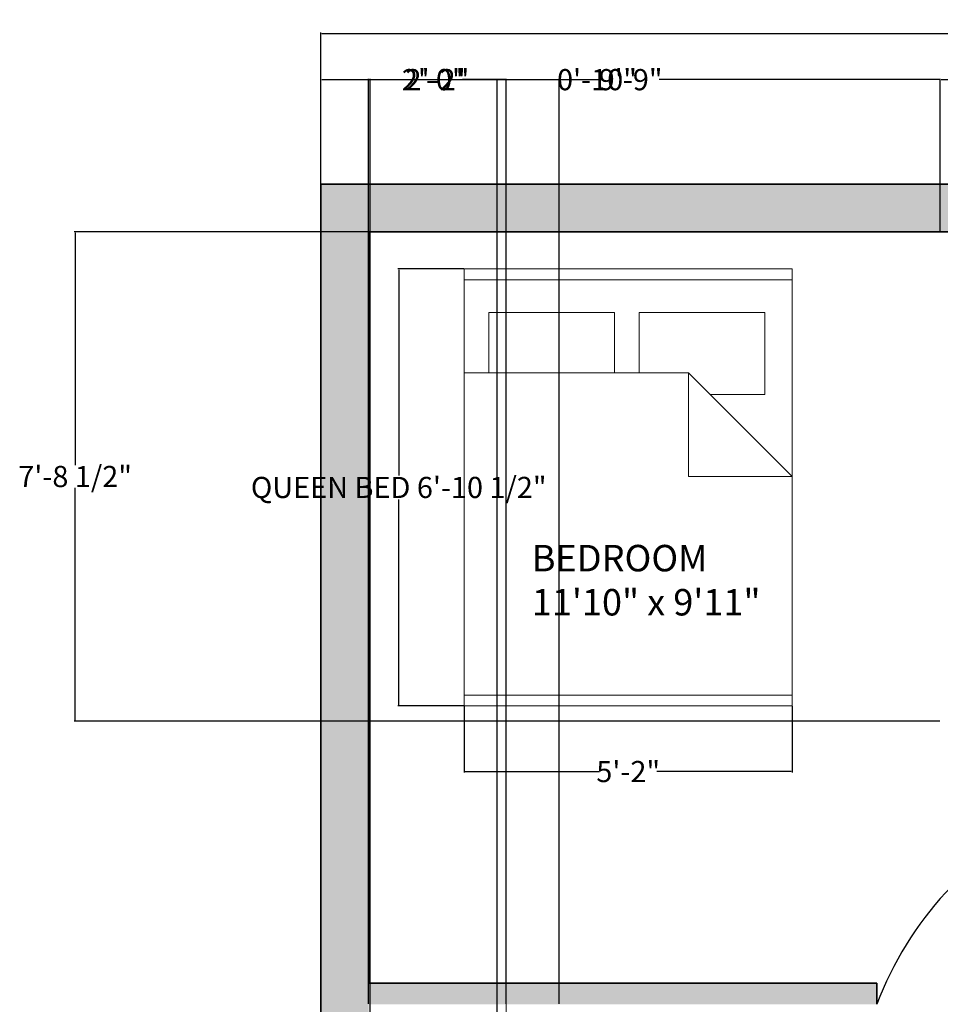
# Model space of a CAD drawing. Units: inches. Extents: x 490 to 851, y 299 to 716.
# Tile 2 of 3: x 490 to 664, y 530 to 716. Entities that reach past the tile are written whole.
import ezdxf

# ---------------------------------------------------------------- set-up
doc = ezdxf.new("R2010")
doc.units = ezdxf.units.IN
doc.header["$MEASUREMENT"] = 0
for name, color, linetype, lineweight in [('A-ANNO-DIMS', 2, 'Continuous', 18), ('A-AREA-IDEN', 7, 'Continuous', 25), ('A-DOOR', 3, 'Continuous', 25), ('A-WALL', 7, 'Continuous', 35), ('A-WALL-PATT', 1, 'Continuous', 13), ('beds', 40, 'Continuous', 18), ('stairs', 82, 'Continuous', 18)]:
    doc.layers.add(name, color=color, linetype=linetype, lineweight=lineweight)
doc.styles.get("Standard").update_dxf_attribs({"font": 'arial.ttf'})
doc.dimstyles.get("Standard").update_dxf_attribs({"dimtxt": 4, "dimasz": 0.18, "dimexe": 0.18, "dimexo": 0.0625, "dimgap": 0.09, "dimtad": 0, "dimtih": 1, "dimtoh": 1, "dimdec": 0, "dimrnd": 6, "dimzin": 0, "dimdsep": 46, "dimlunit": 3, "dimtxsty": 'Standard', "dimcen": 0.09, "dimadec": 0, "dimazin": 0, "dimtfac": 1, "dimtdec": 0, "dimtofl": 0, "dimtmove": 0, "dimatfit": 3, "dimfxl": 1, "dimtolj": 1, "dimtzin": 0, "dimarcsym": 0})

# ---------------------------------------------------------------- blocks, each defined once
blk = doc.blocks.new('QUEEN-00')
for p, q in [((-0.8475, -0.7751), (-0.8475, 0.7489)), ((0.6511, 0.7489), (0.6511, -0.2925)), ((1.0829, 0.7489), (1.0829, -0.7751)), ((0.9305, 0.6346), (0.6511, 0.6346)), ((0.9305, 0.0504), (0.9305, 0.6346)), ((0.6511, 0.0504), (0.9305, 0.0504)), ((0.9305, -0.0639), (0.6511, -0.0639)), ((0.9305, -0.6481), (0.9305, -0.0639)), ((0.1685, -0.7751), (0.6511, -0.2925)), ((0.1685, -0.2925), (0.1685, -0.7751)), ((0.6511, -0.2925), (0.1685, -0.2925)), ((0.5495, -0.3941), (0.5495, -0.6481)), ((0.5495, -0.6481), (0.9305, -0.6481))]:
    blk.add_line(p, q)
blk.add_lwpolyline([(-0.8983, -0.7751), (-0.8983, 0.7489), (1.1337, 0.7489), (1.1337, -0.7751)], close=True)
blk = doc.blocks.new('*D102')
at = {"layer": 'A-ANNO-DIMS', "color": 0, "lineweight": -2, "transparency": 16777216}
for p, q in [((546.69, 685.02), (546.69, 713.6)), ((546.87, 713.42), (681.17, 713.42)), ((822.51, 713.42), (688.21, 713.42)), ((822.69, 685.02), (822.69, 713.6))]:
    blk.add_line(p, q, dxfattribs=at)
at = {"layer": 'A-ANNO-DIMS', "color": 0, "transparency": 16777216}
for points in [[(546.87, 713.45), (546.87, 713.39), (546.69, 713.42)], [(822.51, 713.45), (822.51, 713.39), (822.69, 713.42)]]:
    blk.add_solid(points, dxfattribs=at)
at = {"layer": 'Defpoints', "color": 0, "transparency": 16777216}
for p in [(822.69, 713.42), (546.69, 684.96), (822.69, 684.96)]:
    blk.add_point(p, dxfattribs=at)
at = {"layer": 'A-ANNO-DIMS', "color": 0, "transparency": 16777216, "insert": (684.69, 713.42), "char_height": 4, "attachment_point": 5}
blk.add_mtext("\\A1;23'", dxfattribs=at)
blk = doc.blocks.new('*D112')
at = {"layer": 'A-ANNO-DIMS', "color": 0, "lineweight": -2, "transparency": 16777216}
for p, q in [((573.7, 668.93), (561.2, 668.93)), ((561.38, 668.75), (561.38, 629.92)), ((561.38, 586.52), (561.38, 625.36)), ((573.7, 586.34), (561.2, 586.34))]:
    blk.add_line(p, q, dxfattribs=at)
at = {"layer": 'A-ANNO-DIMS', "color": 0, "transparency": 16777216}
for points in [[(561.35, 668.75), (561.41, 668.75), (561.38, 668.93)], [(561.35, 586.52), (561.41, 586.52), (561.38, 586.34)]]:
    blk.add_solid(points, dxfattribs=at)
at = {"layer": 'Defpoints', "color": 0, "transparency": 16777216}
for p in [(561.38, 668.93), (573.77, 668.93), (573.77, 586.34)]:
    blk.add_point(p, dxfattribs=at)
at = {"layer": 'A-ANNO-DIMS', "color": 0, "transparency": 16777216, "insert": (561.38, 627.64), "char_height": 4, "attachment_point": 5}
blk.add_mtext('\\A1;QUEEN BED 6\'-10 1/2"', dxfattribs=at)
blk = doc.blocks.new('*D113')
at = {"layer": 'A-ANNO-DIMS', "color": 0, "lineweight": -2, "transparency": 16777216}
for p, q in [((573.77, 586.28), (573.77, 573.77)), ((635.71, 586.28), (635.71, 573.77)), ((573.95, 573.95), (599.33, 573.95)), ((635.53, 573.95), (610.15, 573.95))]:
    blk.add_line(p, q, dxfattribs=at)
at = {"layer": 'A-ANNO-DIMS', "color": 0, "transparency": 16777216}
for points in [[(573.95, 573.98), (573.95, 573.92), (573.77, 573.95)], [(635.53, 573.98), (635.53, 573.92), (635.71, 573.95)]]:
    blk.add_solid(points, dxfattribs=at)
at = {"layer": 'Defpoints', "color": 0, "transparency": 16777216}
for p in [(573.77, 586.34), (635.71, 586.34), (573.77, 573.95)]:
    blk.add_point(p, dxfattribs=at)
at = {"layer": 'A-ANNO-DIMS', "color": 0, "transparency": 16777216, "insert": (604.74, 573.95), "char_height": 4, "attachment_point": 5}
blk.add_mtext('\\A1;5\'-2"', dxfattribs=at)
blk = doc.blocks.new('*D122')
at = {"layer": 'A-ANNO-DIMS', "color": 0, "lineweight": -2, "transparency": 16777216}
for p, q in [((546.69, 685.02), (546.69, 704.89)), ((546.87, 704.71), (599.78, 704.71)), ((663.51, 704.71), (610.59, 704.71)), ((663.69, 676.02), (663.69, 704.89))]:
    blk.add_line(p, q, dxfattribs=at)
at = {"layer": 'A-ANNO-DIMS', "color": 0, "transparency": 16777216}
for points in [[(546.87, 704.74), (546.87, 704.68), (546.69, 704.71)], [(663.51, 704.74), (663.51, 704.68), (663.69, 704.71)]]:
    blk.add_solid(points, dxfattribs=at)
at = {"layer": 'Defpoints', "color": 0, "transparency": 16777216}
for p in [(663.69, 704.71), (546.69, 684.96), (663.69, 675.96)]:
    blk.add_point(p, dxfattribs=at)
at = {"layer": 'A-ANNO-DIMS', "color": 0, "transparency": 16777216, "insert": (605.19, 704.71), "char_height": 4, "attachment_point": 5}
blk.add_mtext('\\A1;9\'-9"', dxfattribs=at)
blk = doc.blocks.new('*D123')
at = {"layer": 'A-ANNO-DIMS', "color": 0, "lineweight": -2, "transparency": 16777216}
for p, q in [((663.69, 676.02), (663.69, 704.89)), ((663.87, 704.71), (670.25, 704.71)), ((687.51, 704.71), (681.13, 704.71)), ((687.69, 676.02), (687.69, 704.89))]:
    blk.add_line(p, q, dxfattribs=at)
at = {"layer": 'A-ANNO-DIMS', "color": 0, "transparency": 16777216}
for points in [[(663.87, 704.74), (663.87, 704.68), (663.69, 704.71)], [(687.51, 704.74), (687.51, 704.68), (687.69, 704.71)]]:
    blk.add_solid(points, dxfattribs=at)
at = {"layer": 'Defpoints', "color": 0, "transparency": 16777216}
for p in [(687.69, 704.71), (663.69, 675.96), (687.69, 675.96)]:
    blk.add_point(p, dxfattribs=at)
at = {"layer": 'A-ANNO-DIMS', "color": 0, "transparency": 16777216, "insert": (675.69, 704.71), "char_height": 4, "attachment_point": 5}
blk.add_mtext('\\A1;2\'-0"', dxfattribs=at)
blk = doc.blocks.new('*D125')
at = {"layer": 'A-ANNO-DIMS', "color": 0, "lineweight": -2, "transparency": 16777216}
for p, q in [((663.63, 675.96), (500.07, 675.96)), ((500.25, 675.78), (500.25, 631.87)), ((500.25, 583.64), (500.25, 627.55)), ((663.63, 583.46), (500.07, 583.46))]:
    blk.add_line(p, q, dxfattribs=at)
at = {"layer": 'A-ANNO-DIMS', "color": 0, "transparency": 16777216}
for points in [[(500.22, 675.78), (500.28, 675.78), (500.25, 675.96)], [(500.22, 583.64), (500.28, 583.64), (500.25, 583.46)]]:
    blk.add_solid(points, dxfattribs=at)
at = {"layer": 'Defpoints', "color": 0, "transparency": 16777216}
for p in [(500.25, 675.96), (663.69, 675.96), (663.69, 583.46)]:
    blk.add_point(p, dxfattribs=at)
at = {"layer": 'A-ANNO-DIMS', "color": 0, "transparency": 16777216, "insert": (500.25, 629.71), "char_height": 4, "attachment_point": 5}
blk.add_mtext('\\A1;7\'-8 1/2"', dxfattribs=at)
blk = doc.blocks.new('*D131')
at = {"layer": 'A-ANNO-DIMS', "color": 0, "lineweight": -2, "transparency": 16777216}
for p, q in [((555.69, 530.02), (555.69, 704.89)), ((555.87, 704.71), (563.25, 704.71)), ((581.51, 704.71), (574.13, 704.71)), ((581.69, 530.02), (581.69, 704.89))]:
    blk.add_line(p, q, dxfattribs=at)
at = {"layer": 'A-ANNO-DIMS', "color": 0, "transparency": 16777216}
for points in [[(555.87, 704.74), (555.87, 704.68), (555.69, 704.71)], [(581.51, 704.74), (581.51, 704.68), (581.69, 704.71)]]:
    blk.add_solid(points, dxfattribs=at)
at = {"layer": 'Defpoints', "color": 0, "transparency": 16777216}
for p in [(581.69, 704.71), (555.69, 529.96), (581.69, 529.96)]:
    blk.add_point(p, dxfattribs=at)
at = {"layer": 'A-ANNO-DIMS', "color": 0, "transparency": 16777216, "insert": (568.69, 704.71), "char_height": 4, "attachment_point": 5}
blk.add_mtext('\\A1;2\'-2"', dxfattribs=at)
blk = doc.blocks.new('*D132')
at = {"layer": 'A-ANNO-DIMS', "color": 0, "lineweight": -2, "transparency": 16777216}
for p, q in [((581.69, 530.02), (581.69, 704.89)), ((581.87, 704.71), (591.51, 704.71)), ((591.69, 530.02), (591.69, 704.89)), ((591.69, 704.71), (591.87, 704.71))]:
    blk.add_line(p, q, dxfattribs=at)
at = {"layer": 'A-ANNO-DIMS', "color": 0, "transparency": 16777216}
for points in [[(581.87, 704.74), (581.87, 704.68), (581.69, 704.71)], [(591.51, 704.74), (591.51, 704.68), (591.69, 704.71)]]:
    blk.add_solid(points, dxfattribs=at)
at = {"layer": 'Defpoints', "color": 0, "transparency": 16777216}
for p in [(591.69, 704.71), (581.69, 529.96), (591.69, 529.96)]:
    blk.add_point(p, dxfattribs=at)
at = {"layer": 'A-ANNO-DIMS', "color": 0, "transparency": 16777216, "insert": (598.83, 704.71), "char_height": 4, "attachment_point": 5}
blk.add_mtext('\\A1;0\'-10"', dxfattribs=at)
blk = doc.blocks.new('*D136')
at = {"layer": 'A-ANNO-DIMS', "color": 0, "lineweight": -2, "transparency": 16777216}
for p, q in [((556, 494.66), (556, 704.89)), ((556.18, 704.71), (562.56, 704.71)), ((579.82, 704.71), (573.44, 704.71)), ((580, 490.16), (580, 704.89))]:
    blk.add_line(p, q, dxfattribs=at)
at = {"layer": 'A-ANNO-DIMS', "color": 0, "transparency": 16777216}
for points in [[(556.18, 704.74), (556.18, 704.68), (556, 704.71)], [(579.82, 704.74), (579.82, 704.68), (580, 704.71)]]:
    blk.add_solid(points, dxfattribs=at)
at = {"layer": 'Defpoints', "color": 0, "transparency": 16777216}
for p in [(580, 704.71), (556, 494.6), (580, 490.1)]:
    blk.add_point(p, dxfattribs=at)
at = {"layer": 'A-ANNO-DIMS', "color": 0, "transparency": 16777216, "insert": (568, 704.71), "char_height": 4, "attachment_point": 5}
blk.add_mtext('\\A1;2\'-0"', dxfattribs=at)

msp = doc.modelspace()

# ---------------------------------------------------------------- hatches: boundary and pattern name
at = {"layer": 'A-WALL-PATT'}
h = msp.add_hatch(color=256, dxfattribs=at)
h.dxf.hatch_style = 1
h.paths.add_polyline_path([(555.69, 497.96), (611.69, 497.96), (611.69, 493.96), (615.69, 493.96), (615.69, 501.96), (555.69, 501.96), (555.69, 529.96), (651.69, 529.96), (651.69, 533.96), (555.69, 533.96), (555.69, 675.96), (813.69, 675.96), (813.69, 564.96), (813.69, 560.96), (813.69, 533.96), (802.5, 533.96), (802.5, 529.96), (813.69, 529.96), (813.69, 465.96), (727.69, 465.96), (727.69, 461.96), (813.69, 461.96), (813.69, 333.96), (786.39, 333.96), (786.39, 324.96), (822.69, 324.96), (822.69, 684.96), (546.69, 684.96), (546.69, 324.96), (555.71, 324.96), (555.71, 333.96), (555.69, 333.96), (555.69, 461.96), (651.69, 461.96), (651.69, 465.96), (555.69, 465.96)])
h.paths.add_polyline_path([(714.39, 333.96), (691.69, 333.96), (691.69, 429.92), (691.68, 429.92), (691.68, 465.96), (687.69, 465.96), (687.69, 429.96), (687.69, 361.01), (687.69, 361.01), (687.69, 324.96), (714.39, 324.96)], flags=17)
h.paths.add_polyline_path([(691.69, 675.96), (687.69, 675.96), (687.69, 529.96), (691.69, 529.96)], flags=17)
h.paths.add_polyline_path([(777.76, 533.96), (761.69, 533.96), (761.69, 497.96, -0.03124), (765.69, 498.21), (765.69, 529.96), (777.76, 529.96)], flags=17)
h.paths.add_polyline_path([(777.69, 564.96), (727.69, 564.96), (727.69, 560.96), (777.69, 560.96)], flags=17)

# ---------------------------------------------------------------- linework, layer by layer
at = {"layer": 'A-DOOR'}
msp.add_arc((713.59, 506.39), 66.24, 115.8959, 159.1627, dxfattribs=at)
at = {"layer": 'A-WALL'}
for p, q in [((546.69, 684.96), (546.69, 324.96)), ((822.69, 684.96), (546.69, 684.96)), ((555.69, 675.96), (555.69, 533.96)), ((813.69, 675.96), (555.69, 675.96)), ((651.69, 533.96), (555.69, 533.96)), ((651.69, 533.96), (651.69, 529.96))]:
    msp.add_line(p, q, dxfattribs=at)
at = {"layer": 'stairs'}
msp.add_line((581.69, 529.96), (581.69, 501.96), dxfattribs=at)

# ---------------------------------------------------------------- block references
at = {"layer": 'beds', "xscale": 40.64754459814275, "yscale": 40.64754459814275, "zscale": 40.64754459814275, "rotation": 90}
msp.add_blockref('QUEEN-00', (604.21, 622.85), dxfattribs=at)

# ---------------------------------------------------------------- texts
at = {"layer": 'A-AREA-IDEN', "insert": (586.52, 616.78), "char_height": 5, "attachment_point": 1}
msp.add_mtext_dynamic_manual_height_columns('BEDROOM\\P11\'10" x 9\'11"', width=54.9921, gutter_width=1, heights=[0], dxfattribs=at)

# ---------------------------------------------------------------- dimensions: what is measured, and where the dimension line sits
at = {"layer": 'A-ANNO-DIMS'}
for base, p1, p2, override, picture, middle in [((822.69, 713.42), (546.69, 684.96), (822.69, 684.96), {"dimclrd": 0, "dimclre": 0, "dimclrt": 0}, '*D102', (684.69, 713.42)), ((663.69, 704.71), (546.69, 684.96), (663.69, 675.96), {"dimdec": 1, "dimlfac": 1, "dimrnd": 0, "dimzin": 1, "dimdsep": 46, "dimlunit": 4, "dimfrac": 2}, '*D122', (605.19, 704.71)), ((581.69, 704.71), (555.69, 529.96), (581.69, 529.96), {"dimdec": 1, "dimlfac": 1, "dimrnd": 0, "dimzin": 1, "dimdsep": 46, "dimlunit": 4, "dimfrac": 2}, '*D131', (568.69, 704.71)), ((580, 704.71), (556, 494.6), (580, 490.1), {"dimdec": 1, "dimlfac": 1, "dimrnd": 0, "dimzin": 1, "dimdsep": 46, "dimlunit": 4, "dimfrac": 2}, '*D136', (568, 704.71)), ((591.69, 704.71), (581.69, 529.96), (591.69, 529.96), {"dimdec": 1, "dimlfac": 1, "dimrnd": 0, "dimzin": 1, "dimdsep": 46, "dimlunit": 4, "dimfrac": 2}, '*D132', (598.83, 704.71)), ((687.69, 704.71), (663.69, 675.96), (687.69, 675.96), {"dimdec": 1, "dimlfac": 1, "dimrnd": 0, "dimzin": 1, "dimdsep": 46, "dimlunit": 4, "dimfrac": 2}, '*D123', (675.69, 704.71))]:
    dim = msp.add_linear_dim(base=base, p1=p1, p2=p2, dimstyle='Standard', override=override, dxfattribs=at)
    dim.commit()
    dim.dimension.update_dxf_attribs({"geometry": picture, "text_midpoint": middle})
for base, p1, p2, angle, picture, middle in [((500.25, 675.96), (663.69, 583.46), (663.69, 675.96), 90, '*D125', (500.25, 629.71)), ((573.77, 573.95), (635.71, 586.34), (573.77, 586.34), 180, '*D113', (604.74, 573.95))]:
    dim = msp.add_linear_dim(base=base, p1=p1, p2=p2, angle=angle, dimstyle='Standard', override={"dimdec": 1, "dimlfac": 1, "dimrnd": 0, "dimzin": 1, "dimdsep": 46, "dimlunit": 4, "dimfrac": 2}, dxfattribs=at)
    dim.commit()
    dim.dimension.update_dxf_attribs({"geometry": picture, "text_midpoint": middle})
dim = msp.add_linear_dim(base=(561.38, 668.93), p1=(573.77, 586.34), p2=(573.77, 668.93), angle=90, text='QUEEN BED <>', dimstyle='Standard', override={"dimdec": 1, "dimlfac": 1, "dimrnd": 0, "dimzin": 1, "dimdsep": 46, "dimlunit": 4, "dimfrac": 2}, dxfattribs=at)
dim.commit()
dim.dimension.update_dxf_attribs({"geometry": '*D112', "text_midpoint": (561.38, 627.64)})

doc.saveas('drawing.dxf')
